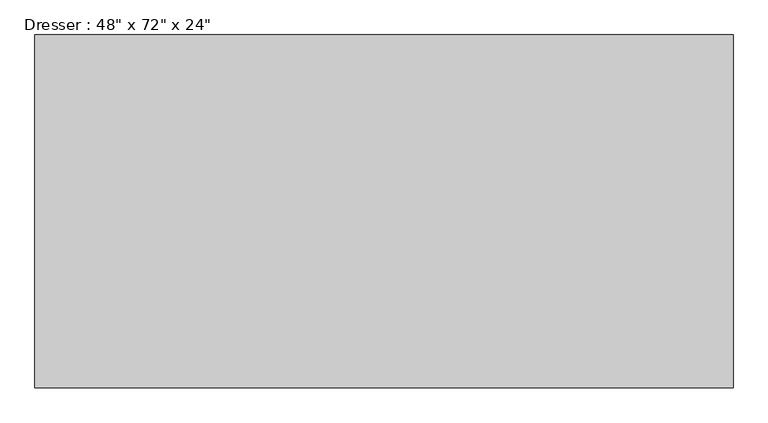
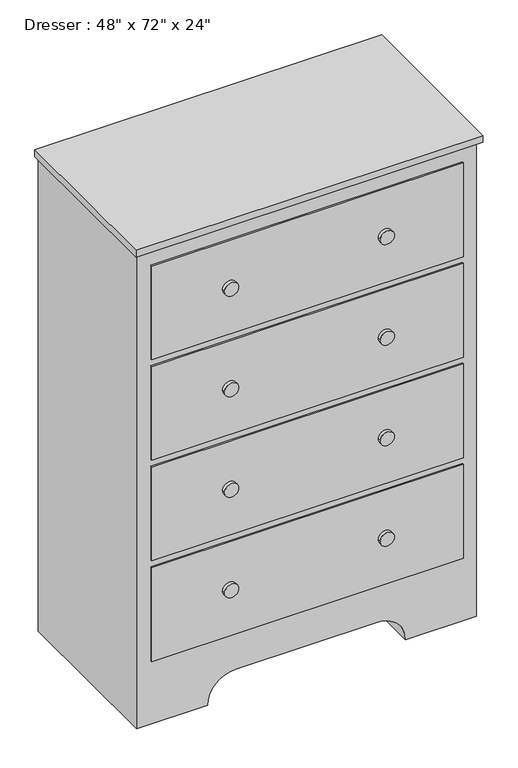
"""IFC4 building model written with IfcOpenShell, lengths in millimetres: furniture geometry."""

from ifc_helpers import new_model, si_unit, point, frame, frame_2d, origin, place, context, project, spatial, polyline, circle_curve, trimmed, segment, composite_curve, outline, extrude, source, transform, mapped, element, save


def furniture_9fa109b2(model_context):
    return source(origin(), model_context, "Body", "SweptSolid", [
        extrude(outline(polyline([(353.1067402, -58.3629541), (353.1067402, -687.0129541), (-891.4932598, -687.0129541), (-891.4932598, -58.3629541), (353.1067402, -58.3629541)])), frame((0.0, 0.0, 1803.4), z_axis=(0.0, 0.0, 1.0), x_axis=(1.0, 0.0, 0.0)), (0.0, 0.0, 1.0), 25.4),
        extrude(outline(composite_curve([segment(polyline([(0.0, 340.4067402), (1803.4, 340.4067402), (1803.4, -878.7932598), (0.0, -878.7932598), (0.0, -624.7932598)]), True, "CONTINUOUS"), segment(trimmed(circle_curve(frame_2d((0.0, -523.1932598)), 101.6), [point((0.0, -624.7932598))], [point((101.6, -523.1932598))], True, "CARTESIAN"), True, "CONTINUOUS"), segment(polyline([(101.6, -523.1932598), (101.6, -15.1932598)]), True, "CONTINUOUS"), segment(trimmed(circle_curve(frame_2d((0.0, -15.1932598)), 101.6), [point((101.6, -15.1932598))], [point((0.0, 86.4067402))], True, "CARTESIAN"), True, "CONTINUOUS"), segment(polyline([(0.0, 86.4067402), (0.0, 340.4067402)]), True, "CONTINUOUS")], self_intersect=False)), frame((0.0, -667.9629541, 0.0), z_axis=(0.0, 1.0, 0.0), x_axis=(0.0, 0.0, 1.0)), (0.0, 0.0, 1.0), 609.6),
        extrude(outline(composite_curve([segment(trimmed(circle_curve(frame_2d((1562.1, 10.2067402)), 25.4), [point((1562.1, -15.1932598))], [point((1562.1, 35.6067402))], False, "CARTESIAN"), True, "CONTINUOUS"), segment(trimmed(circle_curve(frame_2d((1562.1, 10.2067402)), 25.4), [point((1562.1, 35.6067402))], [point((1562.1, -15.1932598))], False, "CARTESIAN"), True, "CONTINUOUS")], self_intersect=False)), frame((0.0, -687.0129541, 0.0), z_axis=(0.0, 1.0, 0.0), x_axis=(0.0, 0.0, 1.0)), (0.0, 0.0, 1.0), 12.7),
        extrude(outline(composite_curve([segment(trimmed(circle_curve(frame_2d((1181.1, 10.2067402)), 25.4), [point((1181.1, -15.1932598))], [point((1181.1, 35.6067402))], False, "CARTESIAN"), True, "CONTINUOUS"), segment(trimmed(circle_curve(frame_2d((1181.1, 10.2067402)), 25.4), [point((1181.1, 35.6067402))], [point((1181.1, -15.1932598))], False, "CARTESIAN"), True, "CONTINUOUS")], self_intersect=False)), frame((0.0, -687.0129541, 0.0), z_axis=(0.0, 1.0, 0.0), x_axis=(0.0, 0.0, 1.0)), (0.0, 0.0, 1.0), 12.7),
        extrude(outline(composite_curve([segment(trimmed(circle_curve(frame_2d((800.1, 10.2067402)), 25.4), [point((800.1, -15.1932598))], [point((800.1, 35.6067402))], False, "CARTESIAN"), True, "CONTINUOUS"), segment(trimmed(circle_curve(frame_2d((800.1, 10.2067402)), 25.4), [point((800.1, 35.6067402))], [point((800.1, -15.1932598))], False, "CARTESIAN"), True, "CONTINUOUS")], self_intersect=False)), frame((0.0, -687.0129541, 0.0), z_axis=(0.0, 1.0, 0.0), x_axis=(0.0, 0.0, 1.0)), (0.0, 0.0, 1.0), 12.7),
        extrude(outline(composite_curve([segment(trimmed(circle_curve(frame_2d((419.1, 10.2067402)), 25.4), [point((419.1, -15.1932598))], [point((419.1, 35.6067402))], False, "CARTESIAN"), True, "CONTINUOUS"), segment(trimmed(circle_curve(frame_2d((419.1, 10.2067402)), 25.4), [point((419.1, 35.6067402))], [point((419.1, -15.1932598))], False, "CARTESIAN"), True, "CONTINUOUS")], self_intersect=False)), frame((0.0, -687.0129541, 0.0), z_axis=(0.0, 1.0, 0.0), x_axis=(0.0, 0.0, 1.0)), (0.0, 0.0, 1.0), 12.7),
        extrude(outline(composite_curve([segment(trimmed(circle_curve(frame_2d((419.1, -548.5932598)), 25.4), [point((419.1, -573.9932598))], [point((419.1, -523.1932598))], False, "CARTESIAN"), True, "CONTINUOUS"), segment(trimmed(circle_curve(frame_2d((419.1, -548.5932598)), 25.4), [point((419.1, -523.1932598))], [point((419.1, -573.9932598))], False, "CARTESIAN"), True, "CONTINUOUS")], self_intersect=False)), frame((0.0, -687.0129541, 0.0), z_axis=(0.0, 1.0, 0.0), x_axis=(0.0, 0.0, 1.0)), (0.0, 0.0, 1.0), 12.7),
        extrude(outline(composite_curve([segment(trimmed(circle_curve(frame_2d((800.1, -548.5932598)), 25.4), [point((800.1, -573.9932598))], [point((800.1, -523.1932598))], False, "CARTESIAN"), True, "CONTINUOUS"), segment(trimmed(circle_curve(frame_2d((800.1, -548.5932598)), 25.4), [point((800.1, -523.1932598))], [point((800.1, -573.9932598))], False, "CARTESIAN"), True, "CONTINUOUS")], self_intersect=False)), frame((0.0, -687.0129541, 0.0), z_axis=(0.0, 1.0, 0.0), x_axis=(0.0, 0.0, 1.0)), (0.0, 0.0, 1.0), 12.7),
        extrude(outline(composite_curve([segment(trimmed(circle_curve(frame_2d((1181.1, -548.5932598)), 25.4), [point((1181.1, -573.9932598))], [point((1181.1, -523.1932598))], False, "CARTESIAN"), True, "CONTINUOUS"), segment(trimmed(circle_curve(frame_2d((1181.1, -548.5932598)), 25.4), [point((1181.1, -523.1932598))], [point((1181.1, -573.9932598))], False, "CARTESIAN"), True, "CONTINUOUS")], self_intersect=False)), frame((0.0, -687.0129541, 0.0), z_axis=(0.0, 1.0, 0.0), x_axis=(0.0, 0.0, 1.0)), (0.0, 0.0, 1.0), 12.7),
        extrude(outline(composite_curve([segment(trimmed(circle_curve(frame_2d((1562.1, -548.5932598)), 25.4), [point((1562.1, -573.9932598))], [point((1562.1, -523.1932598))], False, "CARTESIAN"), True, "CONTINUOUS"), segment(trimmed(circle_curve(frame_2d((1562.1, -548.5932598)), 25.4), [point((1562.1, -523.1932598))], [point((1562.1, -573.9932598))], False, "CARTESIAN"), True, "CONTINUOUS")], self_intersect=False)), frame((0.0, -687.0129541, 0.0), z_axis=(0.0, 1.0, 0.0), x_axis=(0.0, 0.0, 1.0)), (0.0, 0.0, 1.0), 12.7),
        extrude(outline(polyline([(289.6067402, -674.3129541), (-827.9932598, -674.3129541), (-827.9932598, -667.9629541), (289.6067402, -667.9629541), (289.6067402, -674.3129541)])), frame((0.0, 0.0, 1384.3), z_axis=(0.0, 0.0, 1.0), x_axis=(1.0, 0.0, 0.0)), (0.0, 0.0, 1.0), 355.6),
        extrude(outline(polyline([(289.6067402, -674.3129541), (-827.9932598, -674.3129541), (-827.9932598, -667.9629541), (289.6067402, -667.9629541), (289.6067402, -674.3129541)])), frame((0.0, 0.0, 1003.3), z_axis=(0.0, 0.0, 1.0), x_axis=(1.0, 0.0, 0.0)), (0.0, 0.0, 1.0), 355.6),
        extrude(outline(polyline([(289.6067402, -674.3129541), (-827.9932598, -674.3129541), (-827.9932598, -667.9629541), (289.6067402, -667.9629541), (289.6067402, -674.3129541)])), frame((0.0, 0.0, 622.3), z_axis=(0.0, 0.0, 1.0), x_axis=(1.0, 0.0, 0.0)), (0.0, 0.0, 1.0), 355.6),
        extrude(outline(polyline([(289.6067402, -674.3129541), (-827.9932598, -674.3129541), (-827.9932598, -667.9629541), (289.6067402, -667.9629541), (289.6067402, -674.3129541)])), frame((0.0, 0.0, 241.3), z_axis=(0.0, 0.0, 1.0), x_axis=(1.0, 0.0, 0.0)), (0.0, 0.0, 1.0), 355.6),
    ])


if __name__ == "__main__":
    model = new_model("IFC4")
    model_context = context("Model", 3, world=origin())
    ifc_project = project(units=[si_unit("LENGTHUNIT", "METRE", prefix="MILLI")], contexts=[model_context])
    site = spatial("IfcSite", under=ifc_project)
    building = spatial("IfcBuilding", under=site)
    placement = place(None, origin())
    furniture_shape = furniture_9fa109b2(model_context)
    element("IfcFurniture", 1, ObjectType="Dresser : 48\" x 72\" x 24\"", at=placement, inside=building, context=model_context, shape_type="MappedRepresentation", body=[
        mapped(furniture_shape, transform((0.0, 0.0, 0.0), x_axis=(1.0, 0.0, 0.0), y_axis=(0.0, 1.0, 0.0), z_axis=(0.0, 0.0, 1.0))),
    ])
    save(model, "model.ifc")

# Revit data of these elements
# Type "Dresser : 48\" x 72\" x 24\""
#   Assembly Code = "E2020200"
#   Depth = 2' - 0"
#   Height = 6' - 0"
#   Width = 4' - 0"
#   Dresser Material = Wood - Teak
#   Drawer Material = Laminate, Ivory, Matte
#   Knob Material = Cherry
#   Default Elevation = 0
# Element 1 (IfcFurniture, "Dresser : 48\" x 72\" x 24\"")
#   Materials on its faces: "Laminate, Ivory, Matte", "Cherry", "Wood - Teak"
# Materials
#   "Wood - Teak": class "Wood", colour RGB 145 112 90, transparency 0
#   "Laminate, Ivory, Matte": class "Plastic", colour RGB 247 247 239, transparency 0, Description = "Plastic Laminate - Ivory, Matte", Cost = 0
#   "Cherry": class "Wood", colour RGB 226 177 128, transparency 0, Description = "Prunus Serotina", Cost = 0
